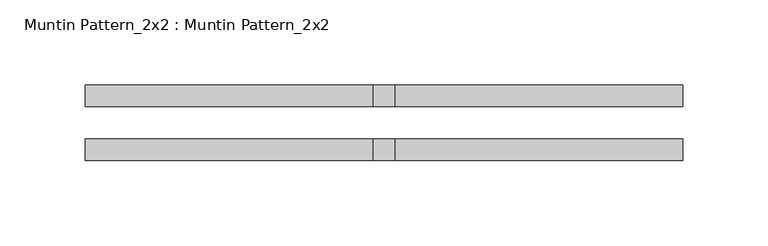
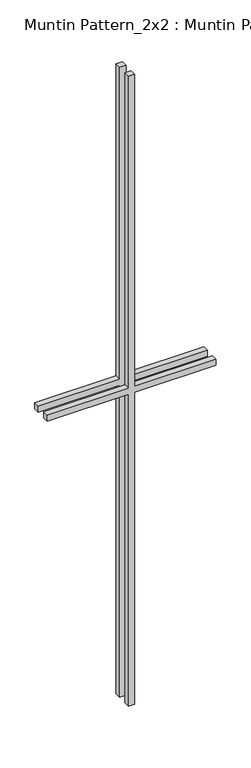
"""IFC4 building model written with IfcOpenShell, lengths in millimetres: proxy geometry, Muntin Pattern_2x2 : Muntin Pattern_2x2."""

from ifc_helpers import new_model, si_unit, frame, origin, place, context, project, spatial, polyline, outline, extrude, source, transform, mapped, element, save


def muntin_pattern_2x2_muntin_pattern_2x2_f815d33b(model_context):
    return source(origin(), model_context, "Body", "SweptSolid", [
        extrude(outline(polyline([(698.5, -6.35), (698.5, -175.7591104), (685.8, -175.7591104), (685.8, -6.35), (0.0, -6.35), (0.0, 6.35), (685.8, 6.35), (685.8, 175.7591104), (698.5, 175.7591104), (698.5, 6.35), (1384.3, 6.35), (1384.3, -6.35), (698.5, -6.35)])), frame((0.0, 9.525, 0.0), z_axis=(0.0, 1.0, 0.0), x_axis=(0.0, 0.0, 1.0)), (0.0, 0.0, 1.0), 12.7),
        extrude(outline(polyline([(698.5, -6.35), (698.5, -175.7591104), (685.8, -175.7591104), (685.8, -6.35), (0.0, -6.35), (0.0, 6.35), (685.8, 6.35), (685.8, 175.7591104), (698.5, 175.7591104), (698.5, 6.35), (1384.3, 6.35), (1384.3, -6.35), (698.5, -6.35)])), frame((0.0, -22.225, 0.0), z_axis=(0.0, 1.0, 0.0), x_axis=(0.0, 0.0, 1.0)), (0.0, 0.0, 1.0), 12.7),
    ])


if __name__ == "__main__":
    model = new_model("IFC4")
    model_context = context("Model", 3, world=origin())
    ifc_project = project(units=[si_unit("LENGTHUNIT", "METRE", prefix="MILLI")], contexts=[model_context])
    site = spatial("IfcSite", under=ifc_project)
    building = spatial("IfcBuilding", under=site)
    placement = place(None, origin())
    muntin_pattern_2x2_muntin_pattern_2x2_shape = muntin_pattern_2x2_muntin_pattern_2x2_f815d33b(model_context)
    element("IfcBuildingElementProxy", 1, Name="Muntin Pattern_2x2 : Muntin Pattern_2x2", ObjectType="Muntin Pattern_2x2 : Muntin Pattern_2x2", at=placement, inside=building, context=model_context, shape_type="MappedRepresentation", body=[
        mapped(muntin_pattern_2x2_muntin_pattern_2x2_shape, transform((0.0, 0.0, 0.0), x_axis=(1.0, 0.0, 0.0), y_axis=(0.0, 1.0, 0.0), z_axis=(0.0, 0.0, 1.0))),
    ])
    save(model, "model.ifc")

# Revit data of these elements
# Type "Muntin Pattern_2x2 : Muntin Pattern_2x2"
#   Width [instance default] = 4' - 0"
#   Thickness = 0' - 0 1/2"
#   Height [instance default] = 4' - 0"
#   Distance = 0' - 0 3/4"
#   Interior Material [instance default] = none
#   Exterior Material [instance default] = none
#   Default Elevation = 0
# Element 1 (IfcBuildingElementProxy, "Muntin Pattern_2x2 : Muntin Pattern_2x2")
#   Width = 1' - 1.8393"
#   Height = 4' - 6 1/2"
#   Interior Material = Wood - Stained
#   Exterior Material = Clad - White
#   Materials on its faces: "Clad - White", "Wood - Stained"
# Materials
#   "Clad - White": class "Wood", colour RGB 242 242 238, transparency 0, Cost = 0
#   "Wood - Stained": class "Wood", colour RGB 224 178 126, transparency 0, Cost = 0
